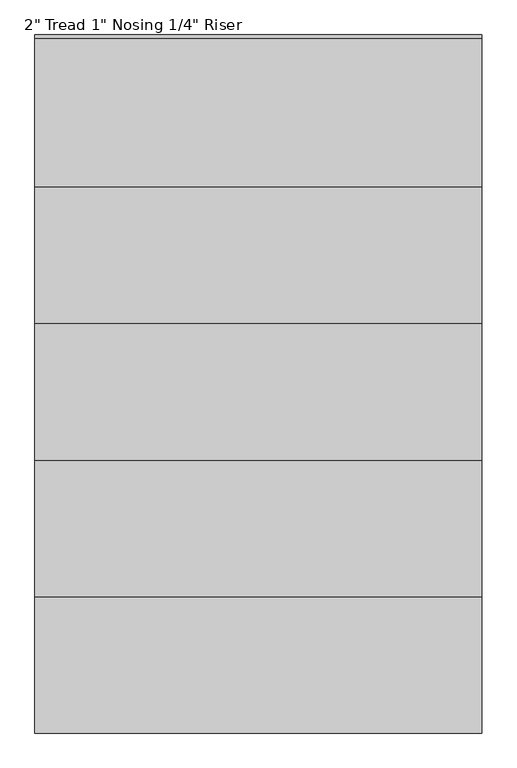
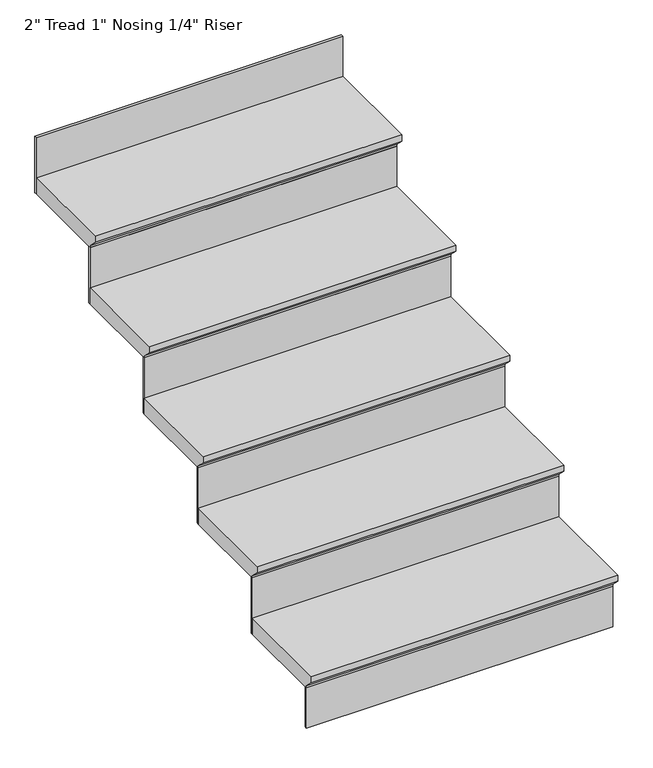
"""IFC4 building model written with IfcOpenShell, lengths in millimetres: stair flight geometry."""

from ifc_helpers import new_model, si_unit, frame, origin, place, context, project, spatial, polyline, outline, extrude, source, transform, mapped, element, save


def stair_flight_a146ff17(model_context):
    return source(origin(), model_context, "Body", "SweptSolid", [
        extrude(outline(polyline([(-2893.1217987, -889.0), (-2588.3217987, -889.0), (-2588.3217987, -939.8), (-2867.7217987, -939.8), (-2867.7217987, -933.45), (-2893.1217987, -908.05), (-2893.1217987, -889.0)])), frame((177.241197, 0.0, 0.0), z_axis=(1.0, 0.0, 0.0), x_axis=(0.0, 1.0, 0.0)), (0.0, 0.0, 1.0), 914.4),
        extrude(outline(polyline([(1091.641197, -2861.3717987), (1091.641197, -2867.7217987), (177.241197, -2867.7217987), (177.241197, -2861.3717987), (1091.641197, -2861.3717987)])), frame((0.0, 0.0, -1066.8), z_axis=(0.0, 0.0, 1.0), x_axis=(1.0, 0.0, 0.0)), (0.0, 0.0, 1.0), 127.0),
        extrude(outline(polyline([(1091.641197, -2581.9717987), (1091.641197, -2588.3217987), (177.241197, -2588.3217987), (177.241197, -2581.9717987), (1091.641197, -2581.9717987)])), frame((0.0, 0.0, -939.8), z_axis=(0.0, 0.0, 1.0), x_axis=(1.0, 0.0, 0.0)), (0.0, 0.0, 1.0), 177.8),
        extrude(outline(polyline([(-2613.7217987, -711.2), (-2308.9217987, -711.2), (-2308.9217987, -762.0), (-2588.3217987, -762.0), (-2588.3217987, -755.65), (-2613.7217987, -730.25), (-2613.7217987, -711.2)])), frame((177.241197, 0.0, 0.0), z_axis=(1.0, 0.0, 0.0), x_axis=(0.0, 1.0, 0.0)), (0.0, 0.0, 1.0), 914.4),
        extrude(outline(polyline([(1091.641197, -2302.5717987), (1091.641197, -2308.9217987), (177.241197, -2308.9217987), (177.241197, -2302.5717987), (1091.641197, -2302.5717987)])), frame((0.0, 0.0, -762.0), z_axis=(0.0, 0.0, 1.0), x_axis=(1.0, 0.0, 0.0)), (0.0, 0.0, 1.0), 177.8),
        extrude(outline(polyline([(-2334.3217987, -533.4), (-2029.5217987, -533.4), (-2029.5217987, -584.2), (-2308.9217987, -584.2), (-2308.9217987, -577.85), (-2334.3217987, -552.45), (-2334.3217987, -533.4)])), frame((177.241197, 0.0, 0.0), z_axis=(1.0, 0.0, 0.0), x_axis=(0.0, 1.0, 0.0)), (0.0, 0.0, 1.0), 914.4),
        extrude(outline(polyline([(1091.641197, -2023.1717987), (1091.641197, -2029.5217987), (177.241197, -2029.5217987), (177.241197, -2023.1717987), (1091.641197, -2023.1717987)])), frame((0.0, 0.0, -584.2), z_axis=(0.0, 0.0, 1.0), x_axis=(1.0, 0.0, 0.0)), (0.0, 0.0, 1.0), 177.8),
        extrude(outline(polyline([(-2054.9217987, -355.6), (-1750.1217987, -355.6), (-1750.1217987, -406.4), (-2029.5217987, -406.4), (-2029.5217987, -400.05), (-2054.9217987, -374.65), (-2054.9217987, -355.6)])), frame((177.241197, 0.0, 0.0), z_axis=(1.0, 0.0, 0.0), x_axis=(0.0, 1.0, 0.0)), (0.0, 0.0, 1.0), 914.4),
        extrude(outline(polyline([(1091.641197, -1743.7717987), (1091.641197, -1750.1217987), (177.241197, -1750.1217987), (177.241197, -1743.7717987), (1091.641197, -1743.7717987)])), frame((0.0, 0.0, -406.4), z_axis=(0.0, 0.0, 1.0), x_axis=(1.0, 0.0, 0.0)), (0.0, 0.0, 1.0), 177.8),
        extrude(outline(polyline([(1091.641197, -1464.3717987), (1091.641197, -1470.7217987), (177.241197, -1470.7217987), (177.241197, -1464.3717987), (1091.641197, -1464.3717987)])), frame((0.0, 0.0, -228.6), z_axis=(0.0, 0.0, 1.0), x_axis=(1.0, 0.0, 0.0)), (0.0, 0.0, 1.0), 177.8),
        extrude(outline(polyline([(-1775.5217987, -177.8), (-1470.7217987, -177.8), (-1470.7217987, -228.6), (-1750.1217987, -228.6), (-1750.1217987, -222.25), (-1775.5217987, -196.85), (-1775.5217987, -177.8)])), frame((177.241197, 0.0, 0.0), z_axis=(1.0, 0.0, 0.0), x_axis=(0.0, 1.0, 0.0)), (0.0, 0.0, 1.0), 914.4),
    ])


if __name__ == "__main__":
    model = new_model("IFC4")
    model_context = context("Model", 3, world=origin())
    ifc_project = project(units=[si_unit("LENGTHUNIT", "METRE", prefix="MILLI")], contexts=[model_context])
    site = spatial("IfcSite", under=ifc_project)
    building = spatial("IfcBuilding", under=site)
    placement = place(None, origin())
    stair_flight_shape = stair_flight_a146ff17(model_context)
    element("IfcStairFlight", 1, ObjectType="2\" Tread 1\" Nosing 1/4\" Riser", at=placement, inside=building, context=model_context, shape_type="MappedRepresentation", body=[
        mapped(stair_flight_shape, transform((0.0, 0.0, 0.0), x_axis=(1.0, 0.0, 0.0), y_axis=(0.0, 1.0, 0.0), z_axis=(0.0, 0.0, 1.0))),
    ])
    save(model, "model.ifc")
